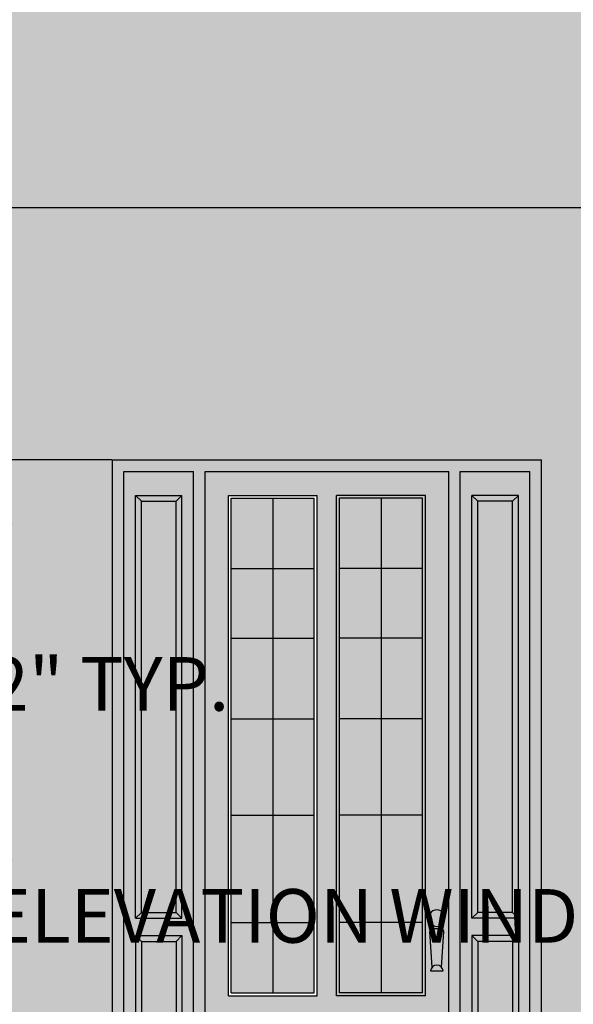
# Model space of a CAD drawing. Units: inches. Extents: x 528 to 2620, y -1066 to 798.
# Tile 38 of 41: x 2384 to 2446, y -1001 to -891. Entities that reach past the tile are written whole.
import ezdxf

# ---------------------------------------------------------------- set-up
doc = ezdxf.new("R2010")
doc.units = ezdxf.units.IN
doc.header["$MEASUREMENT"] = 0
for name, color, linetype, lineweight in [('A-ANNO-DIMS', 2, 'Continuous', 18), ('A-ELEV', 7, 'Continuous', 25), ('A-ELEV-PATT', 8, 'Continuous', 13)]:
    doc.layers.add(name, color=color, linetype=linetype, lineweight=lineweight)
doc.styles.get("Standard").update_dxf_attribs({"font": 'arial.ttf'})
doc.dimstyles.get("Standard").update_dxf_attribs({"dimtxt": 6, "dimasz": 2, "dimexe": 0.18, "dimexo": 0.0625, "dimgap": 0.09, "dimtad": 0, "dimtih": 1, "dimtoh": 1, "dimdec": 1, "dimzin": 0, "dimdsep": 46, "dimlunit": 3, "dimtxsty": 'Standard', "dimblk": 'ARCHTICK', "dimcen": 0.09, "dimadec": 0, "dimazin": 0, "dimtfac": 1, "dimtdec": 1, "dimtofl": 0, "dimtmove": 0, "dimatfit": 3, "dimfxl": 1, "dimtolj": 1, "dimtzin": 0, "dimarcsym": 0})

# ---------------------------------------------------------------- blocks, each defined once
blk = doc.blocks.new('_ArchTick')
at = {"color": 0, "linetype": 'ByBlock', "const_width": 0.15}
blk.add_lwpolyline([(-0.5, -0.5), (0.5, 0.5)], dxfattribs=at)
blk = doc.blocks.new('*D54')
at = {"layer": 'A-ANNO-DIMS', "color": 0, "lineweight": -2, "transparency": 16777216}
for p, q in [((2327.05, -984.21), (2327.05, -991.53)), ((2375.05, -984.21), (2375.05, -991.53)), ((2327.05, -991.35), (2375.05, -991.35)), ((2375.05, -991.35), (2377.05, -991.35))]:
    blk.add_line(p, q, dxfattribs=at)
at = {"layer": 'Defpoints', "color": 0, "transparency": 16777216}
for p in [(2327.05, -984.15), (2375.05, -984.15), (2375.05, -991.35)]:
    blk.add_point(p, dxfattribs=at)
at = {"layer": 'A-ANNO-DIMS', "color": 0, "lineweight": -2, "transparency": 16777216, "xscale": 2, "yscale": 2, "zscale": 2, "rotation": 180}
blk.add_blockref('_ArchTick', (2327.05, -991.35), dxfattribs=at)
at = {"layer": 'A-ANNO-DIMS', "color": 0, "lineweight": -2, "transparency": 16777216, "xscale": 2, "yscale": 2, "zscale": 2}
blk.add_blockref('_ArchTick', (2375.05, -991.35), dxfattribs=at)
at = {"layer": 'A-ANNO-DIMS', "color": 0, "transparency": 16777216, "insert": (2439.5, -991.35), "char_height": 6, "attachment_point": 5}
blk.add_mtext('\\A1;ELEVATION WINDOW 4\'-0" TYP.', dxfattribs=at)
blk = doc.blocks.new('*D55')
at = {"layer": 'A-ANNO-DIMS', "color": 0, "lineweight": -2, "transparency": 16777216}
for p, q in [((2375.11, -946.66), (2382.43, -946.66)), ((2382.25, -946.66), (2382.25, -962.21)), ((2382.25, -984.15), (2382.25, -968.6)), ((2375.11, -984.15), (2382.43, -984.15))]:
    blk.add_line(p, q, dxfattribs=at)
at = {"layer": 'Defpoints', "color": 0, "transparency": 16777216}
for p in [(2375.05, -946.66), (2382.25, -946.66), (2375.05, -984.15)]:
    blk.add_point(p, dxfattribs=at)
at = {"layer": 'A-ANNO-DIMS', "color": 0, "lineweight": -2, "transparency": 16777216, "xscale": 2, "yscale": 2, "zscale": 2}
for p, rotation in [((2382.25, -946.66), 90), ((2382.25, -984.15), 270)]:
    blk.add_blockref('_ArchTick', p, dxfattribs=dict(at, rotation=rotation))
at = {"layer": 'A-ANNO-DIMS', "color": 0, "transparency": 16777216, "insert": (2382.25, -965.41), "char_height": 6, "attachment_point": 5}
blk.add_mtext('\\A1;3\'-1 1/2" TYP.', dxfattribs=at)
blk = doc.blocks.new('*D72')
at = {"layer": 'A-ANNO-DIMS', "color": 0, "lineweight": -2, "transparency": 16777216}
for p, q in [((2394.48, -940.36), (2243.87, -940.36)), ((2244.05, -940.36), (2244.05, -959.1)), ((2244.05, -984.15), (2244.05, -965.41)), ((2326.98, -984.15), (2243.87, -984.15))]:
    blk.add_line(p, q, dxfattribs=at)
at = {"layer": 'Defpoints', "color": 0, "transparency": 16777216}
for p in [(2244.05, -940.36), (2394.55, -940.36), (2327.05, -984.15)]:
    blk.add_point(p, dxfattribs=at)
at = {"layer": 'A-ANNO-DIMS', "color": 0, "lineweight": -2, "transparency": 16777216, "xscale": 2, "yscale": 2, "zscale": 2}
for p, rotation in [((2244.05, -940.36), 90), ((2244.05, -984.15), 270)]:
    blk.add_blockref('_ArchTick', p, dxfattribs=dict(at, rotation=rotation))
at = {"layer": 'A-ANNO-DIMS', "color": 0, "transparency": 16777216, "insert": (2244.05, -962.26), "char_height": 6, "attachment_point": 5}
blk.add_mtext('\\A1;3\'-8"', dxfattribs=at)
blk = doc.blocks.new('*D73')
at = {"layer": 'A-ANNO-DIMS', "color": 0, "lineweight": -2, "transparency": 16777216}
for p, q in [((2265.98, -912.15), (2243.87, -912.15)), ((2244.05, -912.15), (2244.05, -923.15)), ((2244.05, -940.36), (2244.05, -929.36)), ((2394.48, -940.36), (2243.87, -940.36))]:
    blk.add_line(p, q, dxfattribs=at)
at = {"layer": 'Defpoints', "color": 0, "transparency": 16777216}
for p in [(2244.05, -912.15), (2266.05, -912.15), (2394.55, -940.36)]:
    blk.add_point(p, dxfattribs=at)
at = {"layer": 'A-ANNO-DIMS', "color": 0, "lineweight": -2, "transparency": 16777216, "xscale": 2, "yscale": 2, "zscale": 2}
for p, rotation in [((2244.05, -912.15), 90), ((2244.05, -940.36), 270)]:
    blk.add_blockref('_ArchTick', p, dxfattribs=dict(at, rotation=rotation))
at = {"layer": 'A-ANNO-DIMS', "color": 0, "transparency": 16777216, "insert": (2244.05, -926.26), "char_height": 6, "attachment_point": 5}
blk.add_mtext('\\A1;2\'-4"', dxfattribs=at)
blk = doc.blocks.new('*D83')
at = {"layer": 'A-ANNO-DIMS', "color": 0, "lineweight": -2, "transparency": 16777216}
for p, q in [((2375.05, -984.21), (2375.05, -1042.33)), ((2394.55, -1020.21), (2394.55, -1042.33)), ((2375.05, -1042.15), (2394.55, -1042.15)), ((2394.55, -1042.15), (2396.55, -1042.15))]:
    blk.add_line(p, q, dxfattribs=at)
at = {"layer": 'Defpoints', "color": 0, "transparency": 16777216}
for p in [(2375.05, -984.15), (2394.55, -1020.15), (2394.55, -1042.15)]:
    blk.add_point(p, dxfattribs=at)
at = {"layer": 'A-ANNO-DIMS', "color": 0, "lineweight": -2, "transparency": 16777216, "xscale": 2, "yscale": 2, "zscale": 2, "rotation": 180}
blk.add_blockref('_ArchTick', (2375.05, -1042.15), dxfattribs=at)
at = {"layer": 'A-ANNO-DIMS', "color": 0, "lineweight": -2, "transparency": 16777216, "xscale": 2, "yscale": 2, "zscale": 2}
blk.add_blockref('_ArchTick', (2394.55, -1042.15), dxfattribs=at)
at = {"layer": 'A-ANNO-DIMS', "color": 0, "transparency": 16777216, "insert": (2411.32, -1042.15), "char_height": 6, "attachment_point": 5}
blk.add_mtext('\\A1;1\'-7 1/2"', dxfattribs=at)
blk = doc.blocks.new('*D85')
at = {"layer": 'A-ANNO-DIMS', "color": 0, "lineweight": -2, "transparency": 16777216}
for p, q in [((2493.55, -984.21), (2493.55, -1042.33)), ((2442.55, -1020.21), (2442.55, -1042.33)), ((2442.55, -1042.15), (2459.86, -1042.15)), ((2493.55, -1042.15), (2476.23, -1042.15))]:
    blk.add_line(p, q, dxfattribs=at)
at = {"layer": 'Defpoints', "color": 0, "transparency": 16777216}
for p in [(2493.55, -984.15), (2442.55, -1020.15), (2493.55, -1042.15)]:
    blk.add_point(p, dxfattribs=at)
at = {"layer": 'A-ANNO-DIMS', "color": 0, "lineweight": -2, "transparency": 16777216, "xscale": 2, "yscale": 2, "zscale": 2, "rotation": 180}
blk.add_blockref('_ArchTick', (2442.55, -1042.15), dxfattribs=at)
at = {"layer": 'A-ANNO-DIMS', "color": 0, "lineweight": -2, "transparency": 16777216, "xscale": 2, "yscale": 2, "zscale": 2}
blk.add_blockref('_ArchTick', (2493.55, -1042.15), dxfattribs=at)
at = {"layer": 'A-ANNO-DIMS', "color": 0, "transparency": 16777216, "insert": (2468.05, -1042.15), "char_height": 6, "attachment_point": 5}
blk.add_mtext('\\A1;4\'-3"', dxfattribs=at)

msp = doc.modelspace()

# ---------------------------------------------------------------- hatches: boundary and pattern name
at = {"layer": 'A-ELEV-PATT', "transparency": 33554687}
h = msp.add_hatch(color=256, dxfattribs=at)
h.dxf.hatch_style = 1
h.paths.add_polyline_path([(2448.55, -756.15), (2270.55, -756.15), (2270.55, -780.15), (2436.55, -780.15), (2436.55, -888.15), (2266.05, -888.15), (2266.05, -912.15), (2448.55, -912.15)])
h = msp.add_hatch(color=256, dxfattribs=at)
h.dxf.hatch_style = 1
h.paths.add_polyline_path([(2586.55, -912.15), (2448.55, -912.15), (2448.55, -940.66), (2547.55, -940.66), (2547.55, -990.15), (2448.55, -990.15), (2448.55, -1020.15), (2586.55, -1020.15)])
h.paths.add_polyline_path([(2481.55, -789.84), (2562.55, -789.84), (2562.55, -761.55), (2448.55, -761.55), (2448.55, -900.15), (2562.55, -900.15), (2562.55, -876.97), (2481.55, -876.97), (2481.55, -833.41)])
h.paths.add_polyline_path([(2412.55, -780.15), (2298.55, -780.15), (2298.55, -852.15), (2322.55, -852.15), (2322.55, -814.66), (2370.55, -814.66), (2370.55, -852.15), (2412.55, -852.15)])
h.paths.add_polyline_path([(2394.55, -940.36), (2442.55, -940.36), (2442.55, -1020.15), (2448.55, -1020.15), (2448.55, -990.15), (2448.55, -912.15), (2310.55, -912.15), (2310.55, -1020.15), (2394.55, -1020.15)])
h.paths.add_polyline_path([(2327.05, -984.15), (2327.05, -946.66), (2375.05, -946.66), (2375.05, -984.15)], flags=16)
h.paths.add_polyline_path([(2328.71, -982.41), (2328.71, -948.4), (2336.65, -948.4), (2336.73, -948.4), (2373.38, -948.4), (2373.38, -982.41), (2369.7, -982.41)], flags=0)
h.paths.add_polyline_path([(2338.73, -982.41), (2338.73, -948.4), (2351.05, -948.4), (2363.36, -948.4), (2363.36, -982.41), (2351.05, -982.41)], flags=0)
h.paths.add_polyline_path([(2340.4, -980.68), (2340.4, -950.13), (2349.38, -950.13), (2349.38, -980.68)], flags=0)
h.paths.add_polyline_path([(2340.73, -980.33), (2340.73, -950.48), (2349.05, -950.48), (2349.05, -980.33)], flags=0)
h.paths.add_polyline_path([(2352.71, -980.68), (2352.71, -950.13), (2361.7, -950.13), (2361.7, -980.68)], flags=0)
h.paths.add_polyline_path([(2353.05, -980.33), (2353.05, -950.48), (2361.36, -950.48), (2361.36, -980.33)], flags=0)
h.paths.add_polyline_path([(2336.73, -982.41), (2333.05, -982.41), (2333.05, -971.42), (2336.73, -971.42), (2336.73, -970.73), (2333.05, -970.73), (2333.05, -960.08), (2336.73, -960.08), (2336.73, -959.39), (2333.05, -959.39), (2333.05, -948.57), (2336.73, -948.57)], flags=0)
h.paths.add_polyline_path([(2333.22, -982.24), (2333.22, -971.6), (2336.73, -971.6), (2336.73, -982.24)], flags=0)
h.paths.add_polyline_path([(2332.39, -982.41), (2328.71, -982.41), (2328.71, -948.4), (2332.39, -948.4), (2332.39, -959.39), (2328.71, -959.39), (2328.71, -960.08), (2332.39, -960.08), (2332.39, -970.73), (2328.71, -970.73), (2328.71, -971.42), (2332.39, -971.42)], flags=0)
h.paths.add_polyline_path([(2332.22, -982.24), (2328.71, -982.24), (2328.71, -971.6), (2332.22, -971.6)], flags=0)
h.paths.add_polyline_path([(2365.36, -982.41), (2365.36, -948.4), (2369.04, -948.4), (2369.04, -959.39), (2365.36, -959.39), (2365.36, -960.08), (2369.04, -960.08), (2369.04, -970.73), (2365.36, -970.73), (2365.36, -971.42), (2369.04, -971.42), (2369.04, -982.41)], flags=0)
h.paths.add_polyline_path([(2369.7, -971.42), (2373.38, -971.42), (2373.38, -982.24), (2369.7, -982.24)], flags=0)
h.paths.add_polyline_path([(2333.22, -970.55), (2333.22, -960.26), (2336.73, -960.26), (2336.73, -970.55)], flags=0)
h.paths.add_polyline_path([(2332.22, -970.55), (2328.71, -970.55), (2328.71, -960.26), (2332.22, -960.26)], flags=0)
h.paths.add_polyline_path([(2369.7, -970.73), (2369.7, -960.08), (2373.38, -960.08), (2373.38, -970.73)], flags=0)
h.paths.add_polyline_path([(2336.56, -959.22), (2336.56, -948.57), (2336.73, -948.4), (2336.73, -959.22)], flags=0)
h.paths.add_polyline_path([(2332.22, -959.22), (2328.71, -959.22), (2328.71, -948.57), (2332.22, -948.57)], flags=0)
h.paths.add_polyline_path([(2369.7, -959.39), (2369.7, -948.4), (2373.38, -948.4), (2373.38, -959.39)], flags=0)
h = msp.add_hatch(color=256, dxfattribs=at)
h.dxf.hatch_style = 1
h.paths.add_polyline_path([(2403.63, -941.66), (2395.84, -941.66), (2395.84, -1020.15), (2403.63, -1020.15)], flags=17)
h.paths.add_polyline_path([(2402.33, -944.33), (2402.33, -991.61), (2397.14, -991.61), (2397.14, -944.33)], flags=16)
h.paths.add_polyline_path([(2397.79, -944.97), (2401.68, -944.97), (2401.68, -990.96), (2397.79, -990.96)], flags=0)
h.paths.add_polyline_path([(2402.33, -993.55), (2402.33, -1017.32), (2397.14, -1017.32), (2397.14, -993.55)], flags=16)
h.paths.add_polyline_path([(2397.79, -994.2), (2401.68, -994.2), (2401.68, -1016.68), (2397.79, -1016.68)], flags=0)
h.paths.add_polyline_path([(2442.55, -940.36), (2394.55, -940.36), (2394.55, -1020.15), (2395.84, -1020.15), (2395.84, -941.66), (2403.63, -941.66), (2403.63, -1020.15), (2404.92, -1020.15), (2404.92, -941.66), (2432.17, -941.66), (2432.17, -1020.15), (2433.46, -1020.15), (2433.46, -941.66), (2441.25, -941.66), (2441.25, -1020.15), (2442.55, -1020.15)])
h.paths.add_polyline_path([(2432.17, -941.66), (2404.92, -941.66), (2404.92, -1020.15), (2432.17, -1020.15)], flags=17)
h.paths.add_polyline_path([(2417.46, -944.33), (2417.46, -1000.27), (2407.52, -1000.27), (2407.52, -944.33)], flags=16)
h.paths.add_polyline_path([(2417.13, -944.65), (2417.13, -999.95), (2407.84, -999.95), (2407.84, -944.65)], flags=0)
h.paths.add_polyline_path([(2419.63, -944.33), (2429.57, -944.33), (2429.57, -1000.27), (2419.63, -1000.27)], flags=16)
h.paths.add_polyline_path([(2419.96, -944.65), (2429.25, -944.65), (2429.25, -999.95), (2419.96, -999.95)], flags=0)
h.paths.add_polyline_path([(2431.7, -991.59, -1.065994), (2429.97, -991.59, -1.065994)], flags=16)
h.paths.add_polyline_path([(2430.39, -992.77), (2431.28, -992.77, -0.433045), (2431.6, -993.11), (2431.35, -997.08, -0.185872), (2431.53, -997.54), (2430.14, -997.54, -0.185872), (2430.32, -997.08), (2430.06, -993.11, -0.433045)], flags=16)
h.paths.add_polyline_path([(2417.46, -1002.19), (2417.46, -1014.92), (2407.52, -1014.92), (2407.52, -1002.19)], flags=16)
h.paths.add_polyline_path([(2408.82, -1003.49), (2416.16, -1003.49), (2416.16, -1013.62), (2408.82, -1013.62)], flags=0)
h.paths.add_polyline_path([(2419.63, -1002.19), (2429.57, -1002.19), (2429.57, -1014.92), (2419.63, -1014.92)], flags=16)
h.paths.add_polyline_path([(2420.93, -1003.49), (2428.27, -1003.49), (2428.27, -1013.62), (2420.93, -1013.62)], flags=0)
h.paths.add_polyline_path([(2417.13, -944.65), (2412.49, -944.65), (2412.49, -952.52), (2417.13, -952.52)], flags=0)
h.paths.add_polyline_path([(2417.13, -969.31), (2412.49, -969.31), (2412.49, -980.08), (2417.13, -980.08)], flags=0)
h = msp.add_hatch(color=256, dxfattribs=at)
h.dxf.hatch_style = 1
h.paths.add_polyline_path([(2417.13, -969.31), (2412.49, -969.31), (2412.49, -980.08), (2417.13, -980.08)], flags=0)
h.paths.add_polyline_path([(2417.13, -980.08), (2412.49, -980.08), (2412.49, -992.08), (2417.13, -992.08)], flags=0)
h.paths.add_polyline_path([(2412.49, -980.08), (2407.84, -980.08), (2407.84, -992.08), (2412.49, -992.08)], flags=0)
h.paths.add_polyline_path([(2401.68, -944.97), (2397.79, -944.97), (2397.79, -990.96), (2401.68, -990.96)])
h.paths.add_polyline_path([(2401.68, -994.2), (2397.79, -994.2), (2397.79, -1016.68), (2401.68, -1016.68)])
h.paths.add_polyline_path([(2416.16, -1003.49), (2408.82, -1003.49), (2408.82, -1013.62), (2416.16, -1013.62)], flags=0)
h.paths.add_polyline_path([(2428.27, -1003.49), (2420.93, -1003.49), (2420.93, -1013.62), (2428.27, -1013.62)], flags=0)
h.paths.add_polyline_path([(2429.25, -980.08), (2424.6, -980.08), (2424.6, -992.08), (2429.25, -992.08)], flags=0)
h.paths.add_polyline_path([(2424.6, -980.08), (2419.96, -980.08), (2419.96, -992.08), (2424.6, -992.08)], flags=0)
h.paths.add_polyline_path([(2424.6, -992.08), (2419.96, -992.08), (2419.96, -999.95), (2424.6, -999.95)], flags=0)
h.paths.add_polyline_path([(2429.25, -992.08), (2424.6, -992.08), (2424.6, -999.95), (2429.25, -999.95)], flags=0)
h.paths.add_polyline_path([(2417.13, -992.08), (2412.49, -992.08), (2412.49, -999.95), (2417.13, -999.95)], flags=0)
h.paths.add_polyline_path([(2412.49, -992.08), (2407.84, -992.08), (2407.84, -999.95), (2412.49, -999.95)], flags=0)
h.paths.add_polyline_path([(2424.6, -952.52), (2419.96, -952.52), (2419.96, -960.3), (2424.6, -960.3)], flags=0)
h.paths.add_polyline_path([(2424.6, -960.3), (2419.96, -960.3), (2419.96, -969.31), (2424.6, -969.31)], flags=0)
h.paths.add_polyline_path([(2429.25, -960.3), (2424.6, -960.3), (2424.6, -969.31), (2429.25, -969.31)], flags=0)
h.paths.add_polyline_path([(2429.25, -952.52), (2424.6, -952.52), (2424.6, -960.3), (2429.25, -960.3)], flags=0)
h.paths.add_polyline_path([(2429.25, -944.65), (2424.6, -944.65), (2424.6, -952.52), (2429.25, -952.52)], flags=0)
h.paths.add_polyline_path([(2424.6, -944.65), (2419.96, -944.65), (2419.96, -952.52), (2424.6, -952.52)], flags=0)
h.paths.add_polyline_path([(2417.13, -944.65), (2412.49, -944.65), (2412.49, -952.52), (2417.13, -952.52)], flags=0)
h.paths.add_polyline_path([(2412.49, -944.65), (2407.84, -944.65), (2407.84, -952.52), (2412.49, -952.52)], flags=0)
h.paths.add_polyline_path([(2412.49, -952.52), (2407.84, -952.52), (2407.84, -960.3), (2412.49, -960.3)], flags=0)
h.paths.add_polyline_path([(2417.13, -952.52), (2412.49, -952.52), (2412.49, -960.3), (2417.13, -960.3)], flags=0)
h.paths.add_polyline_path([(2432.17, -941.66), (2404.92, -941.66), (2404.92, -1020.15), (2432.17, -1020.15)])
h.paths.add_polyline_path([(2417.46, -944.33), (2417.46, -1000.27), (2407.52, -1000.27), (2407.52, -944.33)], flags=16)
h.paths.add_polyline_path([(2417.13, -944.65), (2417.13, -999.95), (2407.84, -999.95), (2407.84, -944.65)], flags=0)
h.paths.add_polyline_path([(2419.63, -944.33), (2429.57, -944.33), (2429.57, -1000.27), (2419.63, -1000.27)], flags=16)
h.paths.add_polyline_path([(2419.96, -944.65), (2429.25, -944.65), (2429.25, -999.95), (2419.96, -999.95)], flags=0)
h.paths.add_polyline_path([(2431.7, -991.59, -1.065994), (2429.97, -991.59, -1.065994)], flags=16)
h.paths.add_polyline_path([(2430.39, -992.77), (2431.28, -992.77, -0.433045), (2431.6, -993.11), (2431.35, -997.08, -0.185872), (2431.53, -997.54), (2430.14, -997.54, -0.185872), (2430.32, -997.08), (2430.06, -993.11, -0.433045)], flags=16)
h.paths.add_polyline_path([(2417.46, -1002.19), (2417.46, -1014.92), (2407.52, -1014.92), (2407.52, -1002.19)], flags=16)
h.paths.add_polyline_path([(2416.16, -1003.49), (2416.16, -1013.62), (2408.82, -1013.62), (2408.82, -1003.49)], flags=0)
h.paths.add_polyline_path([(2419.63, -1002.19), (2429.57, -1002.19), (2429.57, -1014.92), (2419.63, -1014.92)], flags=16)
h.paths.add_polyline_path([(2420.93, -1003.49), (2428.27, -1003.49), (2428.27, -1013.62), (2420.93, -1013.62)], flags=0)
h.paths.add_polyline_path([(2412.49, -960.3), (2407.84, -960.3), (2407.84, -969.31), (2412.49, -969.31)], flags=0)
h = msp.add_hatch(color=256, dxfattribs=at)
h.dxf.hatch_style = 1
h.paths.add_polyline_path([(2417.13, -980.08), (2412.49, -980.08), (2412.49, -992.08), (2417.13, -992.08)])
h.paths.add_polyline_path([(2412.49, -980.08), (2407.84, -980.08), (2407.84, -992.08), (2412.49, -992.08)])
h.paths.add_polyline_path([(2412.49, -992.08), (2407.84, -992.08), (2407.84, -999.95), (2412.49, -999.95)])
h.paths.add_polyline_path([(2417.13, -992.08), (2412.49, -992.08), (2412.49, -999.95), (2417.13, -999.95)])
h.paths.add_polyline_path([(2424.6, -992.08), (2419.96, -992.08), (2419.96, -999.95), (2424.6, -999.95)])
h.paths.add_polyline_path([(2429.25, -992.08), (2424.6, -992.08), (2424.6, -999.95), (2429.25, -999.95)])
h.paths.add_polyline_path([(2429.25, -980.08), (2424.6, -980.08), (2424.6, -992.08), (2429.25, -992.08)])
h.paths.add_polyline_path([(2424.6, -980.08), (2419.96, -980.08), (2419.96, -992.08), (2424.6, -992.08)])
h.paths.add_polyline_path([(2424.6, -969.31), (2419.96, -969.31), (2419.96, -980.08), (2424.6, -980.08)])
h.paths.add_polyline_path([(2429.25, -969.31), (2424.6, -969.31), (2424.6, -980.08), (2429.25, -980.08)])
h.paths.add_polyline_path([(2424.6, -960.3), (2419.96, -960.3), (2419.96, -969.31), (2424.6, -969.31)])
h.paths.add_polyline_path([(2429.25, -960.3), (2424.6, -960.3), (2424.6, -969.31), (2429.25, -969.31)])
h.paths.add_polyline_path([(2429.25, -952.52), (2424.6, -952.52), (2424.6, -960.3), (2429.25, -960.3)])
h.paths.add_polyline_path([(2424.6, -952.52), (2419.96, -952.52), (2419.96, -960.3), (2424.6, -960.3)])
h.paths.add_polyline_path([(2424.6, -944.65), (2419.96, -944.65), (2419.96, -952.52), (2424.6, -952.52)])
h.paths.add_polyline_path([(2429.25, -944.65), (2424.6, -944.65), (2424.6, -952.52), (2429.25, -952.52)])
h.paths.add_polyline_path([(2417.13, -944.65), (2412.49, -944.65), (2412.49, -952.52), (2417.13, -952.52)])
h.paths.add_polyline_path([(2412.49, -944.65), (2407.84, -944.65), (2407.84, -952.52), (2412.49, -952.52)])
h.paths.add_polyline_path([(2412.49, -952.52), (2407.84, -952.52), (2407.84, -960.3), (2412.49, -960.3)])
h.paths.add_polyline_path([(2417.13, -952.52), (2412.49, -952.52), (2412.49, -960.3), (2417.13, -960.3)])
h.paths.add_polyline_path([(2412.49, -960.3), (2407.84, -960.3), (2407.84, -969.31), (2412.49, -969.31)])
h.paths.add_polyline_path([(2417.13, -960.3), (2412.49, -960.3), (2412.49, -969.31), (2417.13, -969.31)])
h.paths.add_polyline_path([(2412.49, -969.31), (2407.84, -969.31), (2407.84, -980.08), (2412.49, -980.08)])
h.paths.add_polyline_path([(2417.13, -969.31), (2412.49, -969.31), (2412.49, -980.08), (2417.13, -980.08)])
h.paths.add_polyline_path([(2439.3, -994.2), (2435.41, -994.2), (2435.41, -1016.68), (2439.3, -1016.68)], flags=0)
h.paths.add_polyline_path([(2441.25, -941.66), (2433.46, -941.66), (2433.46, -1020.15), (2441.25, -1020.15)])
h.paths.add_polyline_path([(2434.76, -993.55), (2439.95, -993.55), (2439.95, -1017.32), (2434.76, -1017.32)], flags=16)
h.paths.add_polyline_path([(2435.41, -994.2), (2439.3, -994.2), (2439.3, -1016.68), (2435.41, -1016.68)], flags=0)
h.paths.add_polyline_path([(2434.76, -991.61), (2434.76, -944.33), (2439.95, -944.33), (2439.95, -991.61)], flags=16)
h.paths.add_polyline_path([(2435.41, -990.96), (2435.41, -944.97), (2439.3, -944.97), (2439.3, -990.96)], flags=0)
h.paths.add_polyline_path([(2428.27, -1003.49), (2420.93, -1003.49), (2420.93, -1013.62), (2428.27, -1013.62)])
h.paths.add_polyline_path([(2416.16, -1003.49), (2408.82, -1003.49), (2408.82, -1013.62), (2416.16, -1013.62)])
h.paths.add_polyline_path([(2417.46, -1002.19), (2407.52, -1002.19), (2408.82, -1003.49), (2416.16, -1003.49)])
h.paths.add_polyline_path([(2417.46, -1002.19), (2416.16, -1003.49), (2416.16, -1013.62), (2417.46, -1014.92)])
h.paths.add_polyline_path([(2408.82, -1003.49), (2407.52, -1002.19), (2407.52, -1014.92), (2408.82, -1013.62)])
h.paths.add_polyline_path([(2416.16, -1013.62), (2408.82, -1013.62), (2407.52, -1014.92), (2417.46, -1014.92)])
h.paths.add_polyline_path([(2420.93, -1003.49), (2419.63, -1002.19), (2419.63, -1014.92), (2420.93, -1013.62)])
h.paths.add_polyline_path([(2428.27, -1013.62), (2420.93, -1013.62), (2419.63, -1014.92), (2429.57, -1014.92)])
h.paths.add_polyline_path([(2429.57, -1002.19), (2428.27, -1003.49), (2428.27, -1013.62), (2429.57, -1014.92)])
h.paths.add_polyline_path([(2429.57, -1002.19), (2419.63, -1002.19), (2420.93, -1003.49), (2428.27, -1003.49)])
h.paths.add_polyline_path([(2439.3, -944.97), (2435.41, -944.97), (2435.41, -990.96), (2439.3, -990.96)], flags=0)
h = msp.add_hatch(color=256, dxfattribs=at)
h.dxf.hatch_style = 1
h.paths.add_polyline_path([(2424.6, -969.31), (2419.96, -969.31), (2419.96, -980.08), (2424.6, -980.08)])
h.paths.add_polyline_path([(2429.25, -969.31), (2424.6, -969.31), (2424.6, -980.08), (2429.25, -980.08)])
h.paths.add_polyline_path([(2424.6, -980.08), (2419.96, -980.08), (2419.96, -992.08), (2424.6, -992.08)])
h.paths.add_polyline_path([(2429.25, -980.08), (2424.6, -980.08), (2424.6, -992.08), (2429.25, -992.08)])
h.paths.add_polyline_path([(2439.3, -944.97), (2435.41, -944.97), (2435.41, -990.96), (2439.3, -990.96)], flags=0)
h.paths.add_polyline_path([(2435.41, -944.97), (2434.76, -944.33), (2434.76, -991.61), (2435.41, -990.96)], flags=0)
h.paths.add_polyline_path([(2439.3, -990.96), (2435.41, -990.96), (2434.76, -991.61), (2439.95, -991.61)], flags=0)
h.paths.add_polyline_path([(2439.95, -944.33), (2439.3, -944.97), (2439.3, -990.96), (2439.95, -991.61)], flags=0)
h.paths.add_polyline_path([(2441.25, -941.66), (2433.46, -941.66), (2433.46, -1020.15), (2441.25, -1020.15)])
h.paths.add_polyline_path([(2439.95, -991.61), (2434.76, -991.61), (2434.76, -944.33), (2439.95, -944.33)], flags=16)
h.paths.add_polyline_path([(2439.3, -990.96), (2435.41, -990.96), (2435.41, -944.97), (2439.3, -944.97)], flags=0)
h.paths.add_polyline_path([(2439.95, -993.55), (2439.95, -1017.32), (2434.76, -1017.32), (2434.76, -993.55)], flags=16)
h.paths.add_polyline_path([(2439.3, -994.2), (2439.3, -1016.68), (2435.41, -1016.68), (2435.41, -994.2)], flags=0)
h = msp.add_hatch(color=256, dxfattribs=at)
h.dxf.hatch_style = 1
h.paths.add_polyline_path([(2439.3, -944.97), (2435.41, -944.97), (2435.41, -990.96), (2439.3, -990.96)])
h.paths.add_polyline_path([(2439.3, -990.96), (2435.41, -990.96), (2434.76, -991.61), (2439.95, -991.61)])
h.paths.add_polyline_path([(2439.3, -994.2), (2435.41, -994.2), (2435.41, -1016.68), (2439.3, -1016.68)])
h.paths.add_polyline_path([(2439.95, -993.55), (2434.76, -993.55), (2435.41, -994.2), (2439.3, -994.2)])
h.paths.add_polyline_path([(2439.95, -993.55), (2439.3, -994.2), (2439.3, -1016.68), (2439.95, -1017.32)])
h.paths.add_polyline_path([(2435.41, -994.2), (2434.76, -993.55), (2434.76, -1017.32), (2435.41, -1016.68)])
h.paths.add_polyline_path([(2439.3, -1016.68), (2435.41, -1016.68), (2434.76, -1017.32), (2439.95, -1017.32)])
h.paths.add_polyline_path([(2439.95, -944.33), (2434.76, -944.33), (2435.41, -944.97), (2439.3, -944.97)])
h.paths.add_polyline_path([(2401.68, -1016.68), (2397.79, -1016.68), (2397.14, -1017.32), (2402.33, -1017.32)])
h = msp.add_hatch(color=256, dxfattribs=at)
h.dxf.hatch_style = 1
h.paths.add_polyline_path([(2439.3, -944.97), (2435.41, -944.97), (2435.41, -990.96), (2439.3, -990.96)])
h.paths.add_polyline_path([(2439.3, -990.96), (2435.41, -990.96), (2434.76, -991.61), (2439.95, -991.61)])
h.paths.add_polyline_path([(2439.95, -944.33), (2439.3, -944.97), (2439.3, -990.96), (2439.95, -991.61)])
h.paths.add_polyline_path([(2435.41, -944.97), (2434.76, -944.33), (2434.76, -991.61), (2435.41, -990.96)])
h.paths.add_polyline_path([(2439.95, -944.33), (2434.76, -944.33), (2435.41, -944.97), (2439.3, -944.97)])
h.paths.add_polyline_path([(2439.95, -993.55), (2439.3, -994.2), (2439.3, -1016.68), (2439.95, -1017.32)])
h.paths.add_polyline_path([(2439.3, -994.2), (2435.41, -994.2), (2435.41, -1016.68), (2439.3, -1016.68)])
h.paths.add_polyline_path([(2439.3, -1016.68), (2435.41, -1016.68), (2434.76, -1017.32), (2439.95, -1017.32)])
h.paths.add_polyline_path([(2435.41, -994.2), (2434.76, -993.55), (2434.76, -1017.32), (2435.41, -1016.68)])
h.paths.add_polyline_path([(2439.95, -993.55), (2434.76, -993.55), (2435.41, -994.2), (2439.3, -994.2)])
h.paths.add_polyline_path([(2428.27, -1003.49), (2420.93, -1003.49), (2420.93, -1013.62), (2428.27, -1013.62)])
h.paths.add_polyline_path([(2428.27, -1013.62), (2420.93, -1013.62), (2419.63, -1014.92), (2429.57, -1014.92)])
h.paths.add_polyline_path([(2429.57, -1002.19), (2428.27, -1003.49), (2428.27, -1013.62), (2429.57, -1014.92)])
h.paths.add_polyline_path([(2420.93, -1003.49), (2419.63, -1002.19), (2419.63, -1014.92), (2420.93, -1013.62)])
h.paths.add_polyline_path([(2429.57, -1002.19), (2419.63, -1002.19), (2420.93, -1003.49), (2428.27, -1003.49)])
h.paths.add_polyline_path([(2408.82, -1003.49), (2407.52, -1002.19), (2407.52, -1014.92), (2408.82, -1013.62)])
h.paths.add_polyline_path([(2416.16, -1013.62), (2408.82, -1013.62), (2407.52, -1014.92), (2417.46, -1014.92)])
h.paths.add_polyline_path([(2416.16, -1003.49), (2408.82, -1003.49), (2408.82, -1013.62), (2416.16, -1013.62)])
h.paths.add_polyline_path([(2417.46, -1002.19), (2416.16, -1003.49), (2416.16, -1013.62), (2417.46, -1014.92)])
h.paths.add_polyline_path([(2417.46, -1002.19), (2407.52, -1002.19), (2408.82, -1003.49), (2416.16, -1003.49)])
h.paths.add_polyline_path([(2401.68, -994.2), (2397.79, -994.2), (2397.79, -1016.68), (2401.68, -1016.68)])
h.paths.add_polyline_path([(2402.33, -993.55), (2401.68, -994.2), (2401.68, -1016.68), (2402.33, -1017.32)])
h.paths.add_polyline_path([(2401.68, -1016.68), (2397.79, -1016.68), (2397.14, -1017.32), (2402.33, -1017.32)])
h.paths.add_polyline_path([(2397.79, -994.2), (2397.14, -993.55), (2397.14, -1017.32), (2397.79, -1016.68)])
h.paths.add_polyline_path([(2402.33, -993.55), (2397.14, -993.55), (2397.79, -994.2), (2401.68, -994.2)])
h.paths.add_polyline_path([(2412.49, -992.08), (2407.84, -992.08), (2407.84, -999.95), (2412.49, -999.95)])
h.paths.add_polyline_path([(2417.13, -992.08), (2412.49, -992.08), (2412.49, -999.95), (2417.13, -999.95)])
h.paths.add_polyline_path([(2429.25, -992.08), (2424.6, -992.08), (2424.6, -999.95), (2429.25, -999.95)], flags=0)
h.paths.add_polyline_path([(2424.6, -992.08), (2419.96, -992.08), (2419.96, -999.95), (2424.6, -999.95)], flags=0)
h.paths.add_polyline_path([(2417.13, -980.08), (2412.49, -980.08), (2412.49, -992.08), (2417.13, -992.08)])
h.paths.add_polyline_path([(2412.49, -980.08), (2407.84, -980.08), (2407.84, -992.08), (2412.49, -992.08)])
h.paths.add_polyline_path([(2412.49, -969.31), (2407.84, -969.31), (2407.84, -980.08), (2412.49, -980.08)])
h.paths.add_polyline_path([(2417.13, -969.31), (2412.49, -969.31), (2412.49, -980.08), (2417.13, -980.08)])
h.paths.add_polyline_path([(2412.49, -960.3), (2407.84, -960.3), (2407.84, -969.31), (2412.49, -969.31)])
h.paths.add_polyline_path([(2417.13, -960.3), (2412.49, -960.3), (2412.49, -969.31), (2417.13, -969.31)])
h.paths.add_polyline_path([(2412.49, -952.52), (2407.84, -952.52), (2407.84, -960.3), (2412.49, -960.3)])
h.paths.add_polyline_path([(2417.13, -952.52), (2412.49, -952.52), (2412.49, -960.3), (2417.13, -960.3)])
h.paths.add_polyline_path([(2412.49, -944.65), (2407.84, -944.65), (2407.84, -952.52), (2412.49, -952.52)])
h.paths.add_polyline_path([(2417.13, -944.65), (2412.49, -944.65), (2412.49, -952.52), (2417.13, -952.52)])
h.paths.add_polyline_path([(2424.6, -944.65), (2419.96, -944.65), (2419.96, -952.52), (2424.6, -952.52)], flags=0)
h.paths.add_polyline_path([(2429.25, -944.65), (2424.6, -944.65), (2424.6, -952.52), (2429.25, -952.52)], flags=0)
h.paths.add_polyline_path([(2424.6, -952.52), (2419.96, -952.52), (2419.96, -960.3), (2424.6, -960.3)], flags=0)
h.paths.add_polyline_path([(2429.25, -952.52), (2424.6, -952.52), (2424.6, -960.3), (2429.25, -960.3)], flags=0)
h.paths.add_polyline_path([(2424.6, -960.3), (2419.96, -960.3), (2419.96, -969.31), (2424.6, -969.31)], flags=0)
h.paths.add_polyline_path([(2429.25, -960.3), (2424.6, -960.3), (2424.6, -969.31), (2429.25, -969.31)], flags=0)
h.paths.add_polyline_path([(2401.68, -944.97), (2397.79, -944.97), (2397.79, -990.96), (2401.68, -990.96)])
h.paths.add_polyline_path([(2401.68, -990.96), (2397.79, -990.96), (2397.14, -991.61), (2402.33, -991.61)])
h.paths.add_polyline_path([(2402.33, -944.33), (2401.68, -944.97), (2401.68, -990.96), (2402.33, -991.61)])
h.paths.add_polyline_path([(2397.79, -944.97), (2397.14, -944.33), (2397.14, -991.61), (2397.79, -990.96)])
h.paths.add_polyline_path([(2402.33, -944.33), (2397.14, -944.33), (2397.79, -944.97), (2401.68, -944.97)])
h.paths.add_polyline_path([(2429.57, -944.33), (2419.63, -944.33), (2419.63, -1000.27), (2429.57, -1000.27)])
h.paths.add_polyline_path([(2429.25, -999.95), (2419.96, -999.95), (2419.96, -944.65), (2429.25, -944.65)], flags=16)
h = msp.add_hatch(color=256, dxfattribs=at)
h.dxf.hatch_style = 1
h.paths.add_polyline_path([(2424.6, -992.08), (2419.96, -992.08), (2419.96, -999.95), (2424.6, -999.95)])
h.paths.add_polyline_path([(2429.25, -992.08), (2424.6, -992.08), (2424.6, -999.95), (2429.25, -999.95)])
h.paths.add_polyline_path([(2424.6, -960.3), (2419.96, -960.3), (2419.96, -969.31), (2424.6, -969.31)])
h.paths.add_polyline_path([(2429.25, -960.3), (2424.6, -960.3), (2424.6, -969.31), (2429.25, -969.31)])
h.paths.add_polyline_path([(2424.6, -952.52), (2419.96, -952.52), (2419.96, -960.3), (2424.6, -960.3)])
h.paths.add_polyline_path([(2429.25, -952.52), (2424.6, -952.52), (2424.6, -960.3), (2429.25, -960.3)])
h.paths.add_polyline_path([(2424.6, -944.65), (2419.96, -944.65), (2419.96, -952.52), (2424.6, -952.52)])
h.paths.add_polyline_path([(2429.25, -944.65), (2424.6, -944.65), (2424.6, -952.52), (2429.25, -952.52)])
h = msp.add_hatch(color=256, dxfattribs=at)
h.dxf.hatch_style = 1
h.paths.add_polyline_path([(2431.6, -993.11, 0.433045), (2431.28, -992.77), (2430.39, -992.77, 0.433045), (2430.06, -993.11), (2430.32, -997.08, -0.443995), (2431.35, -997.08)])
h.paths.add_polyline_path([(2429.97, -991.59, 1.065994), (2431.7, -991.59, 1.065994)])
h.paths.add_polyline_path([(2430.14, -997.54), (2431.53, -997.54, 1)])
h = msp.add_hatch(color=256, dxfattribs=at)
h.dxf.hatch_style = 1
h.paths.add_polyline_path([(2417.13, -992.08), (2412.49, -992.08), (2412.49, -999.95), (2417.13, -999.95)])

# ---------------------------------------------------------------- linework, layer by layer
at = {"layer": 'A-ELEV'}
for p, q in [((2266.05, -912.15), (2448.55, -912.15)), ((2394.55, -940.36), (2442.55, -940.36)), ((2394.55, -1020.15), (2394.55, -940.36)), ((2442.55, -1020.15), (2442.55, -940.36)), ((2395.84, -1020.15), (2395.84, -941.66)), ((2395.84, -941.66), (2403.63, -941.66)), ((2403.63, -1020.15), (2403.63, -941.66)), ((2404.92, -1020.15), (2404.92, -941.66)), ((2404.92, -941.66), (2432.17, -941.66)), ((2432.17, -1020.15), (2432.17, -941.66)), ((2433.46, -1020.15), (2433.46, -941.66)), ((2433.46, -941.66), (2441.25, -941.66)), ((2441.25, -1020.15), (2441.25, -941.66)), ((2397.14, -991.61), (2397.14, -944.33)), ((2397.14, -944.33), (2402.33, -944.33)), ((2397.79, -944.97), (2397.14, -944.33)), ((2401.68, -944.97), (2402.33, -944.33)), ((2402.33, -991.61), (2402.33, -944.33)), ((2407.52, -1000.27), (2407.52, -944.33)), ((2407.52, -944.33), (2417.46, -944.33)), ((2417.46, -1000.27), (2417.46, -944.33)), ((2419.63, -1000.27), (2419.63, -944.33)), ((2429.57, -944.33), (2419.63, -944.33)), ((2429.57, -1000.27), (2429.57, -944.33)), ((2439.95, -944.33), (2434.76, -944.33)), ((2434.76, -991.61), (2434.76, -944.33)), ((2435.41, -944.97), (2434.76, -944.33)), ((2439.3, -944.97), (2439.95, -944.33)), ((2439.95, -991.61), (2439.95, -944.33)), ((2397.79, -944.97), (2401.68, -944.97)), ((2397.79, -990.96), (2397.79, -944.97)), ((2401.68, -990.96), (2401.68, -944.97)), ((2407.84, -999.95), (2407.84, -944.65)), ((2407.84, -944.65), (2417.13, -944.65)), ((2412.49, -944.65), (2412.49, -999.95)), ((2417.13, -999.95), (2417.13, -944.65)), ((2419.96, -999.95), (2419.96, -944.65)), ((2429.25, -944.65), (2419.96, -944.65)), ((2424.6, -944.65), (2424.6, -999.95)), ((2429.25, -999.95), (2429.25, -944.65)), ((2439.3, -944.97), (2435.41, -944.97)), ((2435.41, -990.96), (2435.41, -944.97)), ((2439.3, -990.96), (2439.3, -944.97)), ((2407.84, -952.52), (2417.13, -952.52)), ((2429.25, -952.52), (2419.96, -952.52)), ((2407.84, -960.3), (2417.13, -960.3)), ((2429.25, -960.3), (2419.96, -960.3)), ((2407.84, -969.31), (2417.13, -969.31)), ((2429.25, -969.31), (2419.96, -969.31)), ((2407.84, -980.08), (2417.13, -980.08)), ((2429.25, -980.08), (2419.96, -980.08)), ((2397.14, -991.61), (2397.79, -990.96)), ((2397.14, -991.61), (2402.33, -991.61)), ((2397.79, -990.96), (2401.68, -990.96)), ((2401.68, -990.96), (2402.33, -991.61)), ((2435.41, -990.96), (2434.76, -991.61)), ((2439.95, -991.61), (2434.76, -991.61)), ((2439.3, -990.96), (2435.41, -990.96)), ((2439.95, -991.61), (2439.3, -990.96)), ((2407.84, -992.08), (2417.13, -992.08)), ((2429.25, -992.08), (2419.96, -992.08)), ((2430.39, -992.77), (2431.28, -992.77)), ((2397.14, -993.55), (2402.33, -993.55)), ((2397.14, -993.55), (2397.14, -1017.32)), ((2397.14, -993.55), (2397.79, -994.2)), ((2401.68, -994.2), (2402.33, -993.55)), ((2402.33, -993.55), (2402.33, -1017.32)), ((2430.32, -997.08), (2430.06, -993.11)), ((2431.35, -997.08), (2431.6, -993.11)), ((2434.76, -993.55), (2434.76, -1017.32)), ((2439.95, -993.55), (2434.76, -993.55)), ((2435.41, -994.2), (2434.76, -993.55)), ((2439.95, -993.55), (2439.3, -994.2)), ((2439.95, -993.55), (2439.95, -1017.32)), ((2397.79, -994.2), (2401.68, -994.2)), ((2397.79, -994.2), (2397.79, -1016.68)), ((2401.68, -994.2), (2401.68, -1016.68)), ((2435.41, -994.2), (2435.41, -1016.68)), ((2439.3, -994.2), (2435.41, -994.2)), ((2439.3, -994.2), (2439.3, -1016.68)), ((2431.53, -997.54), (2430.14, -997.54)), ((2407.52, -1000.27), (2417.46, -1000.27)), ((2407.84, -999.95), (2417.13, -999.95)), ((2429.57, -1000.27), (2419.63, -1000.27)), ((2429.25, -999.95), (2419.96, -999.95))]:
    msp.add_line(p, q, dxfattribs=at)
for centre, radius, start, end in [((2430.83, -991.53), 0.868, 356.3408, 183.6592), ((2430.83, -991.65), 0.868, 176.3408, 3.6592), ((2430.39, -993.09), 0.324, 90, 183.6592), ((2431.28, -993.09), 0.324, 356.3408, 90), ((2430.83, -997.54), 0.695, 0, 180)]:
    msp.add_arc(centre, radius, start, end, dxfattribs=at)

# ---------------------------------------------------------------- dimensions: what is measured, and where the dimension line sits
at = {"layer": 'A-ANNO-DIMS'}
for base, p1, p2, picture, middle in [((2244.05, -912.15), (2394.55, -940.36), (2266.05, -912.15), '*D73', (2244.05, -926.26)), ((2244.05, -940.36), (2327.05, -984.15), (2394.55, -940.36), '*D72', (2244.05, -962.26))]:
    dim = msp.add_linear_dim(base=base, p1=p1, p2=p2, angle=90, dimstyle='Standard', override={"dimdec": 1, "dimlfac": 1, "dimrnd": 0, "dimzin": 1, "dimdsep": 46, "dimlunit": 4, "dimfrac": 2}, dxfattribs=at)
    dim.commit()
    dim.dimension.update_dxf_attribs({"geometry": picture, "text_midpoint": middle})
dim = msp.add_linear_dim(base=(2382.25, -946.66), p1=(2375.05, -984.15), p2=(2375.05, -946.66), angle=90, text='<> TYP.', dimstyle='Standard', override={"dimdec": 1, "dimrnd": 0, "dimzin": 1, "dimlunit": 4, "dimfrac": 2}, dxfattribs=at)
dim.commit()
dim.dimension.update_dxf_attribs({"geometry": '*D55', "text_midpoint": (2382.25, -965.41)})
dim = msp.add_linear_dim(base=(2375.05, -991.35), p1=(2327.05, -984.15), p2=(2375.05, -984.15), text='ELEVATION WINDOW <> TYP.', dimstyle='Standard', override={"dimdec": 1, "dimrnd": 0, "dimzin": 1, "dimlunit": 4, "dimfrac": 2}, dxfattribs=at)
dim.commit()
dim.dimension.update_dxf_attribs({"geometry": '*D54', "text_midpoint": (2439.5, -991.35)})
for base, p1, p2, picture, middle in [((2394.55, -1042.15), (2375.05, -984.15), (2394.55, -1020.15), '*D83', (2411.32, -1042.15)), ((2493.55, -1042.15), (2442.55, -1020.15), (2493.55, -984.15), '*D85', (2468.05, -1042.15))]:
    dim = msp.add_linear_dim(base=base, p1=p1, p2=p2, dimstyle='Standard', override={"dimdec": 1, "dimlfac": 1, "dimrnd": 0, "dimzin": 1, "dimdsep": 46, "dimlunit": 4, "dimfrac": 2}, dxfattribs=at)
    dim.commit()
    dim.dimension.update_dxf_attribs({"geometry": picture, "text_midpoint": middle})

doc.saveas('drawing.dxf')
